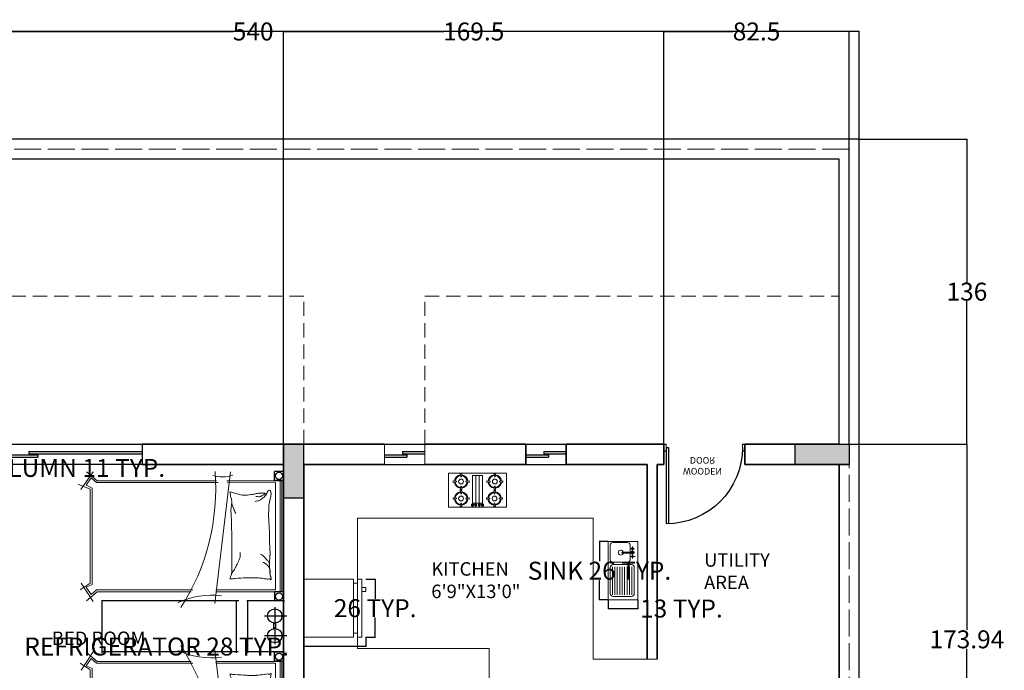
# Model space of a CAD drawing. Units: inches. Extents: x -48 to 50072, y 0 to 21068.
# Tile 71 of 75: x 925 to 1363, y 1005 to 1295. Entities that reach past the tile are written whole.
import ezdxf

# ---------------------------------------------------------------- set-up
doc = ezdxf.new("R2010")
doc.units = ezdxf.units.IN
doc.header["$MEASUREMENT"] = 0
doc.linetypes.add('ACAD_ISO02W100', pattern=[15, 12, -3])
doc.linetypes.add('HIDDEN', pattern=[9.525, 6.35, -3.175])
for name, color, linetype, lineweight in [('A-ANNO-DIMS', 2, 'Continuous', 18), ('A-AREA-IDEN', 7, 'Continuous', 18), ('A-COLS', 1, 'Continuous', 35), ('A-DOOR', 4, 'Continuous', 18), ('A-EQPM', 8, 'Continuous', 18), ('A-FLOR-CASE', 9, 'Continuous', 18), ('A-FLOR-FIXT', 4, 'Continuous', 18), ('A-FLOR-OVHD', 8, 'HIDDEN', 13), ('A-GLAZ', 4, 'Continuous', 18), ('A-WALL', 7, 'Continuous', 35), ('C-PROP', 7, 'Continuous', 25), ('C-PROP-REF', 32, 'ACAD_ISO02W100', 13), ('FURNITURE', 44, 'Continuous', 18)]:
    doc.layers.add(name, color=color, linetype=linetype, lineweight=lineweight)
for name, color, linetype in [('Layer3', 176, 'Continuous'), ('家具1', 1, 'Continuous'), ('家具１', 1, 'Continuous')]:
    doc.layers.add(name, color=color, linetype=linetype)
doc.styles.get("Standard").update_dxf_attribs({"font": 'arial.ttf'})
doc.dimstyles.get("Standard").update_dxf_attribs({"dimtxt": 8, "dimasz": 0.18, "dimexe": 0.18, "dimexo": 0.0625, "dimgap": 0.09, "dimtad": 0, "dimtih": 1, "dimtoh": 1, "dimdec": 1, "dimzin": 0, "dimdsep": 46, "dimlunit": 4, "dimtxsty": 'Standard', "dimblk": 'ARCHTICK', "dimcen": 0.09, "dimadec": 0, "dimazin": 0, "dimtfac": 1, "dimtdec": 1, "dimtofl": 0, "dimtmove": 0, "dimatfit": 3, "dimldrblk": 'ARCHTICK', "dimfxl": 1, "dimtolj": 1, "dimtzin": 0, "dimarcsym": 0})

# ---------------------------------------------------------------- blocks, each defined once
blk = doc.blocks.new('sliding')
blk.add_line((137.02, 1025.77), (137.02, 1034.77))
at = {"layer": 'Defpoints'}
for p, q in [((183.57, 1031.47), (234.12, 1031.47)), ((183.57, 1031.47), (183.57, 1030.47)), ((234.12, 1034.77), (234.12, 1025.77)), ((137.02, 1030.07), (187.57, 1030.07)), ((137.02, 1029.07), (187.57, 1029.07)), ((183.57, 1030.47), (234.12, 1030.47)), ((187.57, 1030.07), (187.57, 1029.07))]:
    blk.add_line(p, q, dxfattribs=at)
at = {"layer": 'Layer3'}
for p, q in [((137.02, 1034.77), (234.12, 1034.77)), ((234.12, 1025.77), (137.02, 1025.77))]:
    blk.add_line(p, q, dxfattribs=at)
blk = doc.blocks.new('bnniku')
at = {"layer": 'Defpoints'}
h = blk.add_hatch(color=256, dxfattribs=at)
h.dxf.hatch_style = 1
h.paths.add_polyline_path([(767.55, 1114.04), (758.55, 1114.04), (758.55, 1090.04), (767.55, 1090.04)])
for p, q in [((758.55, 1114.04), (767.55, 1114.04)), ((758.55, 1090.04), (758.55, 1114.04)), ((767.55, 1114.04), (767.55, 1090.04)), ((767.55, 1090.04), (758.55, 1090.04))]:
    blk.add_line(p, q, dxfattribs=at)
blk = doc.blocks.new('jyugcli')
for p, q in [((342.02, 1025.77), (342.02, 1034.77)), ((360.02, 1025.77), (360.02, 1034.77))]:
    blk.add_line(p, q)
at = {"layer": 'Defpoints'}
for p, q in [((350.02, 1031.47), (360.02, 1031.47)), ((350.02, 1031.47), (350.02, 1030.47)), ((342.02, 1030.07), (352.02, 1030.07)), ((342.02, 1029.07), (352.02, 1029.07)), ((350.02, 1030.47), (360.02, 1030.47)), ((352.02, 1030.07), (352.02, 1029.07))]:
    blk.add_line(p, q, dxfattribs=at)
at = {"layer": 'Layer3'}
for p, q in [((342.02, 1034.77), (360.02, 1034.77)), ((342.02, 1025.77), (360.02, 1025.77))]:
    blk.add_line(p, q, dxfattribs=at)
blk = doc.blocks.new('BKUHJKKUG')
at = {"layer": 'Defpoints'}
for p, q in [((179.52, 862.77), (179.52, 896.77)), ((180.52, 862.77), (180.52, 896.76)), ((179.52, 862.77), (180.52, 862.77))]:
    blk.add_line(p, q, dxfattribs=at)
blk.add_arc((179.52, 862.77), 34, 0, 90, dxfattribs=at)
at = {"insert": (190.84, 874.8), "char_height": 2.9183, "attachment_point": 1}
blk.add_mtext_dynamic_manual_height_columns('\\pxqc;WOODEN ^JDOOR', width=9.6242, gutter_width=14.59, heights=[0], dxfattribs=at)
blk = doc.blocks.new('yfhjudru')
for p, q in [((399.02, 912.27), (399.02, 916.77)), ((435.02, 912.27), (435.02, 916.77)), ((400.02, 912.27), (400.02, 915.27)), ((434.02, 912.27), (434.02, 915.27))]:
    blk.add_line(p, q)
at = {"layer": 'Defpoints'}
for p, q in [((399.02, 915.27), (400.02, 915.27)), ((434.02, 915.27), (435.02, 915.27)), ((399.02, 912.27), (400.02, 912.27)), ((434.02, 912.27), (435.02, 912.27))]:
    blk.add_line(p, q, dxfattribs=at)
blk.add_blockref('BKUHJKKUG', (220.5, 51), dxfattribs=at)
blk = doc.blocks.new('A$C7A8469D8')
for p, q in [((105, 2275), (1345, 2275)), ((105, 1661), (105, 2275)), ((1345, 2255), (105, 2255)), ((1325, 2205), (125, 2205)), ((129, 1663), (125, 2205)), ((1325, 1539), (1325, 2205)), ((1345, 2275), (1345, 1540)), ((3364, 2275), (2124, 2275)), ((2124, 2275), (2124, 1540)), ((2124, 2255), (3364, 2255)), ((2144, 2205), (3344, 2205)), ((2144, 1539), (2144, 2205)), ((3340, 1663), (3344, 2205)), ((3364, 1661), (3364, 2275)), ((997, 2116), (997, 2116)), ((2472, 2116), (2472, 2116)), ((284, 2013), (284, 2013)), ((284, 2013), (284, 2013)), ((941, 2062), (941, 2062)), ((964, 2087), (964, 2087)), ((964, 2087), (964, 2087)), ((2506, 2087), (2506, 2087)), ((2506, 2087), (2506, 2087)), ((2528, 2062), (2528, 2062)), ((3185, 2013), (3185, 2013)), ((3185, 2013), (3185, 2013)), ((240, 1733), (265, 1832)), ((1065, 1762), (1065, 1762)), ((2405, 1762), (2405, 1762)), ((3229, 1733), (3205, 1832)), ((1476, 1525), (6, 1701)), ((231, 1697), (230, 1695)), ((231, 1697), (240, 1733)), ((1097, 1744), (1097, 1744)), ((1097, 1744), (1097, 1744)), ((1097, 1744), (1097, 1744)), ((1993, 1525), (3463, 1701)), ((2372, 1744), (2372, 1744)), ((2372, 1744), (2372, 1744)), ((2372, 1744), (2372, 1744)), ((3238, 1697), (3229, 1733)), ((3238, 1697), (3239, 1695)), ((105, 212), (105, 1543)), ((125, 205), (125, 1562)), ((3344, 205), (3344, 1562)), ((3364, 212), (3364, 1543)), ((1325, 205), (1325, 1280)), ((1345, 1261), (1345, 212)), ((2124, 1261), (2124, 212)), ((2144, 205), (2144, 1280)), ((4, 94), (105, 212)), ((204, 30), (7, 169)), ((125, 205), (73, 144)), ((73, 144), (155, 88)), ((199, 135), (142, 0)), ((155, 88), (187, 155)), ((187, 155), (1264, 155)), ((1251, 135), (199, 135)), ((1453, 169), (1249, 34)), ((1324, 21), (1251, 135)), ((1296, 88), (1264, 155)), ((1378, 144), (1296, 88)), ((1325, 205), (1378, 144)), ((1345, 212), (1446, 92)), ((2017, 169), (2221, 34)), ((2124, 212), (2023, 92)), ((2144, 205), (2092, 144)), ((2092, 144), (2173, 88)), ((2145, 21), (2218, 135)), ((2173, 88), (2205, 155)), ((3282, 155), (2205, 155)), ((2218, 135), (3270, 135)), ((3265, 30), (3463, 169)), ((3270, 135), (3328, 0)), ((3315, 88), (3282, 155)), ((3396, 144), (3315, 88)), ((3344, 205), (3396, 144)), ((3465, 94), (3364, 212))]:
    blk.add_line(p, q)
for centre, radius, start, end in [((227, 2136), 15.7, 101.2724, 206.5805), ((250, 2148), 41, 206.5805, 265.5998), ((245, 2045), 108, 90, 101.2724), ((833, 2043), 590, 173.7676, 180), ((245, 1961), 193, 81.5628, 90), ((170, 1957), 168, 45.0976, 62.7964), ((220, 1790), 366, 74.256, 81.5628), ((398, 2422), 291, 254.256, 262.4531), ((468, 2946), 819, 262.4531, 270), ((468, 3385), 1259, 270, 276.0867), ((201, 24611), 22481, 271.0184, 271.708), ((904, 1960), 183, 92.5386, 100.1899), ((911, 1796), 348, 85.1982, 92.5386), ((1028, 3186), 1048, 265.1982, 269.4243), ((1289, 1747), 470, 128.3886, 133.8115), ((1289, 1747), 470, 128.3886, 133.8115), ((1289, 1747), 470, 128.3886, 133.8115), ((1054, 2044), 92.1, 117.2396, 128.3886), ((1141, 1876), 281, 110.8603, 117.2396), ((1035, 3931), 1793, 269.4243, 271.9079), ((1130, 2026), 119, 143.8234, 161.5603), ((1130, 2026), 119, 126.0864, 143.8234), ((1130, 2026), 119, 105.9352, 126.0864), ((1062, 3124), 985, 271.9079, 275.2592), ((1130, 2026), 119, 85.7841, 105.9352), ((1147, 2207), 64.7, 275.2592, 300.6513), ((1197, 2122), 34.7, 85.6975, 120.6513), ((1434, 2041), 238, 167.8905, 172.3191), ((1198, 2126), 30.1, 68.2117, 85.6975), ((1220, 2138), 18.7, 158.0096, 201.421), ((912, 2153), 295, 347.8905, 351.8665), ((1207, 2143), 5.13, 78.1069, 158.0096), ((1166, 2117), 39.3, 351.8665, 21.421), ((1209, 2151), 2.78, 258.1069, 19.564), ((1207, 2150), 4.1, 19.564, 68.2117), ((2257, 2156), 4.1, 291.7883, 340.436), ((2259, 2149), 2.78, 340.436, 101.8931), ((2258, 2184), 30.1, 274.3025, 291.7883), ((2266, 2150), 5.13, 201.9904, 281.8931), ((2228, 2126), 39.3, 338.579, 8.1335), ((1976, 2049), 295, 8.1335, 12.1095), ((2284, 2138), 18.7, 158.579, 201.9904), ((2504, 2123), 238, 187.6809, 192.1095), ((2287, 2186), 34.7, 239.3487, 274.3025), ((2284, 2087), 64.7, 59.3487, 84.7408), ((2284, 1158), 985, 84.7408, 88.0921), ((2363, 2260), 119, 254.0648, 274.2159), ((2442, 2237), 119, 233.9136, 254.0648), ((2392, 346), 1793, 88.0921, 90.5757), ((2505, 2193), 119, 216.1766, 233.9136), ((2557, 2388), 281, 242.7604, 249.1397), ((2548, 2134), 119, 198.4397, 216.1766), ((2540, 1094), 1048, 90.5757, 94.8018), ((2514, 2198), 92.1, 231.6114, 242.7604), ((2798, 2455), 470, 226.1885, 231.6114), ((2180, 1747), 470, 46.1885, 51.6114), ((2180, 1747), 470, 46.1885, 51.6114), ((2544, 2489), 348, 267.4614, 274.8018), ((2606, 2323), 183, 259.8101, 267.4614), ((2198, -20338), 22481, 88.292, 88.9816), ((2868, 875), 1259, 83.9133, 90), ((3109, 1314), 819, 90, 97.5469), ((3188, 1854), 291, 97.5469, 105.744), ((3096, 2504), 366, 278.4372, 285.744), ((3104, 2226), 168, 297.2036, 314.9024), ((3196, 2345), 193, 270, 278.4372), ((3259, 2088), 41, 94.4002, 153.4195), ((3813, 2107), 590, 180, 186.2324), ((3245, 2260), 108, 258.7276, 270), ((3259, 2145), 15.7, 153.4195, 258.7276), ((488, 2043), 245, 180, 189.6844), ((181, 2001), 108, 41.4429, 53.7359), ((1290, 2180), 1058, 189.6844, 192.1984), ((214, 2030), 63.1, 25.3551, 41.4429), ((108, 1980), 181, 21.8149, 25.3551), ((47, 1955), 247, 18.7799, 21.8149), ((217, 2013), 67.4, 0, 18.7799), ((174, 2013), 110, 345.3149, 360), ((170, 1957), 168, 27.3988, 45.0976), ((170, 1957), 168, 16.515, 27.3988), ((170, 1957), 168, 5.6311, 16.515), ((1146, 1939), 240, 151.6832, 156.9972), ((987, 2024), 59.2, 140.9651, 151.6832), ((1151, 1892), 270, 133.8115, 140.9651), ((1151, 1892), 270, 133.8115, 140.9651), ((1151, 1892), 270, 133.8115, 140.9651), ((2003, 1943), 814, 176.6313, 181.6331), ((2284, 1927), 1096, 172.3191, 176.6313), ((3365, 2137), 1096, 183.3687, 187.6809), ((3094, 1968), 814, 178.3669, 183.3687), ((2716, 2257), 270, 219.0349, 226.1885), ((2319, 1892), 270, 39.0349, 46.1885), ((2319, 1892), 270, 39.0349, 46.1885), ((2581, 2090), 59.2, 208.3168, 219.0349), ((2756, 2146), 240, 203.0028, 208.3168), ((2972, 2022), 168, 343.485, 354.3689), ((2990, 2082), 168, 332.6012, 343.485), ((3032, 2154), 168, 314.9024, 332.6012), ((3121, 2035), 67.4, 341.2201, 360), ((3079, 1985), 110, 0, 14.6851), ((2960, 2126), 247, 338.1851, 341.2201), ((3030, 2125), 181, 334.6449, 338.1851), ((3151, 2099), 63.1, 318.5571, 334.6449), ((3144, 2159), 108, 306.2641, 318.5571), ((4257, 1778), 1058, 167.8016, 170.3156), ((3468, 2002), 245, 170.3156, 180), ((-117, 1876), 381, 8.0051, 12.1984), ((-523, 1819), 791, 2.6649, 8.0051), ((2826, 1967), 1638, 181.6331, 183.055), ((17530, 2751), 16363, 183.055, 183.5049), ((18611, 879), 16363, 176.4951, 176.945), ((3917, 1833), 1638, 176.945, 178.3669), ((2419, 1966), 791, 351.9949, 357.3351), ((2837, 2009), 381, 347.8016, 351.9949), ((186, 1852), 81.3, 345.9548, 2.6649), ((93, 2561), 886, 293.4844, 295.3111), ((927, 1484), 326, 85.9172, 93.5552), ((946, 1740), 69.6, 69.3257, 85.9172), ((755, 1236), 608, 65.6735, 69.3257), ((298, 224), 1719, 63.5015, 65.6735), ((897, 1427), 375, 57.865, 63.5015), ((897, 1427), 375, 57.865, 63.5015), ((897, 1427), 375, 57.865, 63.5015), ((2205, 2080), 375, 296.4985, 302.135), ((2572, 1427), 375, 116.4985, 122.135), ((2572, 1427), 375, 116.4985, 122.135), ((1697, 3328), 1719, 294.3265, 296.4985), ((2249, 2359), 608, 290.6743, 294.3265), ((2494, 1874), 69.6, 274.0828, 290.6743), ((2539, 2135), 326, 266.4448, 274.0828), ((2644, 947), 886, 64.6889, 66.5156), ((3123, 1836), 81.3, 357.3351, 14.0452), ((-288, 1612), 350, 341.9888, 19.1136), ((209, 2020), 325, 273.8155, 274.0829), ((232, 1697), 1.1, 165.9546, 274.0829), ((232, 1697), 1.1, 165.9551, 274.0829), ((209, 2020), 325, 274.0829, 279.4841), ((217, 1971), 276, 279.4841, 287.3864), ((342, 1571), 144, 96.4341, 107.3864), ((346, 1540), 175, 78.4414, 96.4341), ((93, 2561), 886, 287.1982, 289.428), ((436, 1982), 276, 258.4414, 272.7491), ((93, 2561), 886, 289.4267, 291.8864), ((93, 2561), 886, 289.4283, 291.559), ((93, 2561), 886, 289.428, 291.6577), ((93, 2561), 886, 289.4267, 289.4283), ((93, 2561), 886, 291.443, 291.8345), ((93, 2561), 886, 291.43, 291.71), ((93, 2561), 886, 291.43, 291.7259), ((93, 2561), 886, 291.443, 291.484), ((93, 2561), 886, 291.484, 291.7259), ((93, 2561), 886, 291.559, 291.8345), ((93, 2561), 886, 291.6577, 293.4844), ((93, 2561), 886, 291.71, 291.8864), ((369, 3390), 1686, 272.7491, 274.6176), ((622, 254), 1460, 92.6096, 94.6176), ((1098, -33471), 35188, 90.3285, 90.8836), ((1012, -5145), 6862, 89.7135, 90.9704), ((1040, 320), 1397, 86.426, 89.7135), ((632, 1004), 874, 54.1737, 57.865), ((1116, 1540), 175, 77.131, 86.426), ((1143, 1657), 54.3, 62.7159, 77.131), ((1210, 1788), 92.1, 242.7159, 253.7788), ((1214, 1800), 105, 253.7788, 262.8796), ((1582, 1775), 385, 183.5049, 189.9984), ((1201, 1697), 1.59, 262.8796, 343.3022), ((1180, 1704), 23.2, 343.3022, 9.9984), ((2651, 1684), 385, 170.0016, 176.4951), ((2244, 1701), 23.2, 350.0016, 16.6978), ((2267, 1695), 1.59, 16.6978, 97.1204), ((2298, 1595), 105, 97.1204, 106.2212), ((2327, 1617), 92.1, 106.2212, 117.2841), ((2289, 1759), 54.3, 282.869, 297.2841), ((2303, 1885), 175, 273.574, 282.869), ((1861, 2453), 874, 302.135, 305.8263), ((2335, 3111), 1397, 270.2865, 273.574), ((2539, 8578), 6862, 269.0296, 270.2865), ((3116, 36900), 35188, 269.1164, 269.6715), ((3031, 3168), 1460, 265.3824, 267.3904), ((2884, 26), 1686, 85.3824, 87.2509), ((3075, 1435), 276, 87.2509, 101.5586), ((2696, 925), 886, 66.5156, 68.3423), ((3376, 2561), 886, 248.1136, 250.5733), ((3376, 2561), 886, 248.1136, 248.29), ((3376, 2561), 886, 248.1655, 248.557), ((3376, 2561), 886, 248.1655, 248.441), ((3376, 2561), 886, 248.29, 248.57), ((3376, 2561), 886, 248.2741, 248.57), ((3376, 2561), 886, 248.2741, 248.516), ((2754, 902), 886, 68.3423, 70.572), ((3376, 2561), 886, 248.441, 250.5717), ((3376, 2561), 886, 248.516, 248.557), ((3376, 2561), 886, 250.5717, 250.5733), ((2819, 879), 886, 70.572, 72.8018), ((3108, 1885), 175, 263.5659, 281.5586), ((3186, 1851), 144, 252.6136, 263.5659), ((3125, 1436), 276, 72.6136, 80.5159), ((3184, 1375), 325, 80.5159, 85.9171), ((3237, 1697), 1.1, 265.9171, 14.0454), ((3238, 1696), 1.1, 85.9171, 194.0449), ((3260, 2020), 325, 265.9171, 266.1845), ((3757, 1612), 350, 160.8864, 198.0112), ((2297, 1493), 913, 173.1442, 204.7336), ((1172, 1493), 913, 335.2664, 6.8558), ((192, -937), 2473, 57.4247, 94.4416), ((3278, -937), 2473, 85.5584, 122.5753)]:
    blk.add_arc(centre, radius, start, end)
at = {"layer": '家具1'}
for p, q in [((1614, 2082), (1614, 2330)), ((1836, 2082), (1836, 2330)), ((101, 2293), (1, 2293)), ((1, 2293), (1, 2193)), ((101, 2293), (101, 2193)), ((1348, 2293), (1448, 2293)), ((1348, 2293), (1348, 2193)), ((2032, 2293), (1441, 2293)), ((1448, 2303), (1448, 1885)), ((1448, 2293), (1448, 2193)), ((1757, 2206), (1696, 2206)), ((2018, 2303), (2018, 1885)), ((2121, 2293), (2021, 2293)), ((2021, 2293), (2021, 2193)), ((2121, 2293), (2121, 2193)), ((3369, 2293), (3469, 2293)), ((3369, 2293), (3369, 2193)), ((101, 2193), (1, 2193)), ((1348, 2193), (1448, 2193)), ((1518, 2197), (1709, 2197)), ((1757, 2186), (1696, 2186)), ((1741, 2197), (1931, 2197)), ((2121, 2193), (2021, 2193)), ((3369, 2193), (3469, 2193)), ((2029, 1893), (1441, 1893)), ((2029, 1768), (1441, 1768)), ((1448, 1793), (1448, 260)), ((2018, 1788), (2018, 260)), ((2029, 268), (1441, 268))]:
    blk.add_line(p, q, dxfattribs=at)
for centre, radius in [((51, 2243), 40), ((1398, 2243), 40), ((1616, 2196), 80), ((1836, 2196), 80), ((2071, 2243), 40), ((3419, 2243), 40)]:
    blk.add_circle(centre, radius, dxfattribs=at)
at = {"layer": '家具１'}
blk.add_line((3469, 2293), (3469, 2193), dxfattribs=at)
blk = doc.blocks.new('A$C593E77E4')
for p, q in [((0, 0), (0, 0.911)), ((0, 0.911), (1.781, 0.911)), ((1.781, 0), (1.781, 0.911)), ((0.321, 0.668), (0.105, 0.668)), ((0.279, 0.745, -0.922), (0.15, 0.745, -0.922)), ((0.216, 0.808, -0.922), (0.216, 0.672, -0.922)), ((0.321, 0.784, -0.922), (0.321, 0.434, -0.922)), ((0.349, 0.784, -0.922), (0.321, 0.784, -0.922)), ((0.349, 0.434, -0.922), (0.349, 0.784, -0.922)), ((0.555, 0.668), (0.349, 0.668)), ((0.39, 0.745, -0.922), (0.519, 0.745, -0.922)), ((0.455, 0.826, -0.922), (0.455, 0.689, -0.922)), ((0.705, 0.706), (0.705, 0.158)), ((0.772, 0.729, 1.373), (1.625, 0.729, 1.373)), ((0.772, 0.654, 1.373), (1.625, 0.654, 1.373)), ((1.588, 0.797), (0.797, 0.797)), ((1.68, 0.158), (1.68, 0.706)), ((0.03, 0.593), (0.03, 0.141)), ((0.63, 0.141), (0.63, 0.593)), ((0.772, 0.579, 1.373), (1.625, 0.579, 1.373)), ((0.772, 0.504, 1.373), (1.625, 0.504, 1.373)), ((0.772, 0.429, 1.373), (1.625, 0.429, 1.373)), ((0.772, 0.354, 1.373), (1.625, 0.354, 1.373)), ((0.105, 0.066), (0.555, 0.066)), ((0.772, 0.279, 1.373), (1.625, 0.279, 1.373)), ((0.772, 0.204, 1.373), (1.625, 0.204, 1.373)), ((0.772, 0.129, 1.373), (1.625, 0.129, 1.373)), ((0.797, 0.066), (1.588, 0.066)), ((1.781, 0), (0, 0))]:
    blk.add_line(p, q)
for centre in [(0.216, 0.745, -0.922), (0.454, 0.745, -0.922)]:
    blk.add_circle(centre, 0.0299)
for centre, radius, start, end in [((0.105, 0.593), 0.075, 90, 180), ((0.333, 0.75, -0.922), 0.0447, 290.1713, 253.9866), ((0.555, 0.593), 0.075, 0, 90), ((0.797, 0.706), 0.0919, 90, 180), ((1.588, 0.706), 0.0919, 0, 90), ((0.336, 0.387, 0.688), 0.0774, 101.239, 83.3158), ((0.335, 0.435, -0.922), 0.0139, 185.1203, 354.8797), ((0.105, 0.141), 0.075, 180, 270), ((0.555, 0.141), 0.075, 270, 0), ((0.797, 0.158), 0.0919, 180, 270), ((1.588, 0.158), 0.0919, 270, 0)]:
    blk.add_arc(centre, radius, start, end)
blk = doc.blocks.new('A$C57CF26DA')
for p, q in [((0, 0), (0, 420)), ((720, 420), (0, 420)), ((167, 413), (147, 413)), ((147, 413), (152, 373)), ((152, 373), (162, 373)), ((162, 373), (167, 413)), ((300, 391), (300, 49)), ((300, 391), (420, 391)), ((340, 391), (340, 49)), ((380, 391), (380, 49)), ((420, 391), (420, 49)), ((584, 413), (564, 413)), ((564, 413), (569, 373)), ((569, 373), (579, 373)), ((579, 373), (584, 413)), ((720, 0), (720, 420)), ((99, 320), (59, 325)), ((59, 325), (59, 305)), ((59, 305), (99, 310)), ((99, 310), (99, 320)), ((152, 257), (147, 217)), ((162, 257), (152, 257)), ((167, 217), (162, 257)), ((255, 325), (215, 320)), ((215, 320), (215, 310)), ((215, 310), (255, 305)), ((255, 305), (255, 325)), ((516, 320), (476, 325)), ((476, 325), (476, 305)), ((476, 305), (516, 310)), ((516, 310), (516, 320)), ((569, 257), (564, 217)), ((579, 257), (569, 257)), ((584, 217), (579, 257)), ((672, 325), (632, 320)), ((632, 320), (632, 310)), ((632, 310), (672, 305)), ((672, 305), (672, 325)), ((147, 217), (167, 217)), ((167, 203), (147, 203)), ((147, 203), (152, 163)), ((152, 163), (162, 163)), ((162, 163), (167, 203)), ((581, 203), (561, 203)), ((561, 203), (566, 163)), ((564, 217), (584, 217)), ((566, 163), (576, 163)), ((576, 163), (581, 203)), ((99, 110), (59, 115)), ((59, 115), (59, 95)), ((59, 95), (99, 100)), ((99, 100), (99, 110)), ((152, 47), (147, 7)), ((147, 7), (167, 7)), ((162, 47), (152, 47)), ((167, 7), (162, 47)), ((255, 115), (215, 110)), ((215, 110), (215, 100)), ((215, 100), (255, 95)), ((255, 95), (255, 115)), ((302, 39), (295, 39)), ((295, 39), (295, 11)), ((295, 11), (302, 11)), ((420, 49), (300, 49)), ((302, 11), (302, 39)), ((341, 39), (334, 39)), ((334, 39), (334, 11)), ((334, 11), (341, 11)), ((341, 11), (341, 39)), ((380, 11), (380, 39)), ((380, 39), (386, 39)), ((386, 11), (380, 11)), ((386, 39), (386, 11)), ((419, 11), (419, 39)), ((419, 39), (426, 39)), ((426, 11), (419, 11)), ((426, 39), (426, 11)), ((513, 110), (473, 115)), ((473, 115), (473, 95)), ((473, 95), (513, 100)), ((513, 100), (513, 110)), ((566, 47), (561, 7)), ((561, 7), (581, 7)), ((576, 47), (566, 47)), ((581, 7), (576, 47)), ((669, 115), (629, 110)), ((629, 110), (629, 100)), ((629, 100), (669, 95)), ((669, 95), (669, 115)), ((720, 0), (0, 0))]:
    blk.add_line(p, q)
for centre in [(157, 315), (574, 315), (157, 105), (571, 105)]:
    blk.add_circle(centre, 30)
for centre, radius, start, end in [((157, 315), 83, 95.5849, 174.4151), ((157, 315), 73, 95.3738, 174.6262), ((157, 315), 73, 5.3738, 84.6262), ((157, 315), 83, 5.5849, 84.4151), ((574, 315), 83, 95.5849, 174.4151), ((574, 315), 73, 95.3738, 174.6262), ((574, 315), 73, 5.3738, 84.6262), ((574, 315), 83, 5.5849, 84.4151), ((157, 315), 83, 185.5849, 264.4151), ((157, 315), 73, 185.3738, 264.6262), ((157, 315), 73, 275.3738, 354.6262), ((157, 315), 83, 275.5849, 354.4151), ((574, 315), 83, 185.5849, 264.4151), ((574, 315), 73, 185.3738, 264.6262), ((574, 315), 73, 275.3738, 354.6262), ((574, 315), 83, 275.5849, 354.4151), ((157, 105), 83, 95.5849, 174.4151), ((157, 105), 73, 95.3738, 174.6262), ((157, 105), 73, 5.3738, 84.6262), ((157, 105), 83, 5.5849, 84.4151), ((571, 105), 83, 95.5849, 174.4151), ((571, 105), 73, 95.3738, 174.6262), ((571, 105), 73, 5.3738, 84.6262), ((571, 105), 83, 5.5849, 84.4151), ((157, 105), 83, 185.5849, 264.4151), ((157, 105), 73, 185.3738, 264.6262), ((157, 105), 73, 275.3738, 354.6262), ((157, 105), 83, 275.5849, 354.4151), ((298, 25), 13.7, 104.4775, 255.5225), ((298, 25), 13.7, 284.4775, 75.5225), ((337, 25), 13.7, 104.4775, 255.5225), ((337, 25), 13.7, 284.4775, 75.5225), ((383, 25), 13.7, 104.4775, 255.5225), ((383, 25), 13.7, 284.4775, 75.5225), ((422, 25), 13.7, 104.4775, 255.5225), ((422, 25), 13.7, 284.4775, 75.5225), ((571, 105), 83, 185.5849, 264.4151), ((571, 105), 73, 185.3738, 264.6262), ((571, 105), 73, 275.3738, 354.6262), ((571, 105), 83, 275.5849, 354.4151)]:
    blk.add_arc(centre, radius, start, end)
blk = doc.blocks.new('REFRI-00')
for points in [[(-0.35, 0.35), (-0.35, -0.25), (0.35, -0.25), (0.35, 0.35), (-0.35, 0.35)], [(-0.35, -0.3), (-0.35, -0.35), (0.35, -0.35), (0.35, -0.3), (-0.35, -0.3)], [(-0.3, -0.3), (-0.3, -0.25)], [(-0.25, -0.35), (-0.25, -0.4), (-0.2, -0.4), (-0.2, -0.35)], [(0.3, -0.3), (0.3, -0.25)]]:
    blk.add_lwpolyline(points)
blk = doc.blocks.new('_ArchTick')
at = {"color": 0, "linetype": 'ByBlock', "const_width": 0.15}
blk.add_lwpolyline([(-0.5, -0.5), (0.5, 0.5)], dxfattribs=at)
blk = doc.blocks.new('*D50')
at = {"layer": 'A-ANNO-DIMS', "color": 0, "lineweight": -2, "transparency": 16777216}
for p, q in [((850.76, 1096.4), (850.76, 1094.71)), ((850.76, 1094.89), (861.26, 1094.89)), ((861.26, 1096.4), (861.26, 1094.71)), ((861.26, 1094.89), (861.44, 1094.89))]:
    blk.add_line(p, q, dxfattribs=at)
at = {"layer": 'Defpoints', "color": 0, "transparency": 16777216}
for p in [(850.76, 1096.46), (861.26, 1096.46), (861.26, 1094.89)]:
    blk.add_point(p, dxfattribs=at)
at = {"layer": 'A-ANNO-DIMS', "color": 0, "lineweight": -2, "transparency": 16777216, "xscale": 0.18, "yscale": 0.18, "zscale": 0.18, "rotation": 180}
blk.add_blockref('_ArchTick', (850.76, 1094.89), dxfattribs=at)
at = {"layer": 'A-ANNO-DIMS', "color": 0, "lineweight": -2, "transparency": 16777216, "xscale": 0.18, "yscale": 0.18, "zscale": 0.18}
blk.add_blockref('_ArchTick', (861.26, 1094.89), dxfattribs=at)
at = {"layer": 'A-ANNO-DIMS', "color": 0, "transparency": 16777216, "insert": (927.86, 1094.89), "char_height": 8, "attachment_point": 5}
blk.add_mtext('\\A1;SHORT COLUMN 11 TYP.', dxfattribs=at)
blk = doc.blocks.new('*D88')
at = {"layer": 'A-ANNO-DIMS', "color": 0, "lineweight": -2, "transparency": 16777216}
for p, q in [((1186.84, 1062.05), (1182.84, 1062.05)), ((1183.02, 1062.05), (1183.02, 1053.31)), ((1183.02, 1036.11), (1183.02, 1044.85)), ((1186.84, 1036.11), (1182.84, 1036.11))]:
    blk.add_line(p, q, dxfattribs=at)
at = {"layer": 'Defpoints', "color": 0, "transparency": 16777216}
for p in [(1186.91, 1062.05), (1183.02, 1036.11), (1186.91, 1036.11)]:
    blk.add_point(p, dxfattribs=at)
at = {"layer": 'A-ANNO-DIMS', "color": 0, "lineweight": -2, "transparency": 16777216, "xscale": 0.18, "yscale": 0.18, "zscale": 0.18}
for p, rotation in [((1183.02, 1062.05), 90), ((1183.02, 1036.11), 270)]:
    blk.add_blockref('_ArchTick', p, dxfattribs=dict(at, rotation=rotation))
at = {"layer": 'A-ANNO-DIMS', "color": 0, "transparency": 16777216, "insert": (1183.02, 1049.08), "char_height": 8, "attachment_point": 5}
blk.add_mtext('\\A1;SINK 26 TYP.', dxfattribs=at)
blk = doc.blocks.new('*D89')
at = {"layer": 'A-ANNO-DIMS', "color": 0, "lineweight": -2, "transparency": 16777216}
for p, q in [((1186.91, 1036.05), (1186.91, 1032.04)), ((1200.16, 1036.05), (1200.16, 1032.04)), ((1186.91, 1032.22), (1200.16, 1032.22)), ((1200.16, 1032.22), (1200.34, 1032.22))]:
    blk.add_line(p, q, dxfattribs=at)
at = {"layer": 'Defpoints', "color": 0, "transparency": 16777216}
for p in [(1186.91, 1036.11), (1200.16, 1036.11), (1200.16, 1032.22)]:
    blk.add_point(p, dxfattribs=at)
at = {"layer": 'A-ANNO-DIMS', "color": 0, "lineweight": -2, "transparency": 16777216, "xscale": 0.18, "yscale": 0.18, "zscale": 0.18, "rotation": 180}
blk.add_blockref('_ArchTick', (1186.91, 1032.22), dxfattribs=at)
at = {"layer": 'A-ANNO-DIMS', "color": 0, "lineweight": -2, "transparency": 16777216, "xscale": 0.18, "yscale": 0.18, "zscale": 0.18}
blk.add_blockref('_ArchTick', (1200.16, 1032.22), dxfattribs=at)
at = {"layer": 'A-ANNO-DIMS', "color": 0, "transparency": 16777216, "insert": (1219.53, 1032.22), "char_height": 8, "attachment_point": 5}
blk.add_mtext('\\A1;13 TYP.', dxfattribs=at)
blk = doc.blocks.new('*D92')
at = {"layer": 'A-ANNO-DIMS', "color": 0, "lineweight": -2, "transparency": 16777216}
for p, q in [((1051.25, 1019.39), (1051.25, 1015.11)), ((1078.96, 1019.39), (1078.96, 1015.11)), ((1051.25, 1015.29), (1051.07, 1015.29)), ((1078.96, 1015.29), (1051.25, 1015.29))]:
    blk.add_line(p, q, dxfattribs=at)
at = {"layer": 'Defpoints', "color": 0, "transparency": 16777216}
for p in [(1051.25, 1019.45), (1078.96, 1019.45), (1051.25, 1015.29)]:
    blk.add_point(p, dxfattribs=at)
at = {"layer": 'A-ANNO-DIMS', "color": 0, "lineweight": -2, "transparency": 16777216, "xscale": 0.18, "yscale": 0.18, "zscale": 0.18, "rotation": 180}
blk.add_blockref('_ArchTick', (1051.25, 1015.29), dxfattribs=at)
at = {"layer": 'A-ANNO-DIMS', "color": 0, "lineweight": -2, "transparency": 16777216, "xscale": 0.18, "yscale": 0.18, "zscale": 0.18}
blk.add_blockref('_ArchTick', (1078.96, 1015.29), dxfattribs=at)
at = {"layer": 'A-ANNO-DIMS', "color": 0, "transparency": 16777216, "insert": (985.76, 1015.29), "char_height": 8, "attachment_point": 5}
blk.add_mtext('\\A1;REFRIGERATOR 28 TYP.', dxfattribs=at)
blk = doc.blocks.new('*D93')
at = {"layer": 'A-ANNO-DIMS', "color": 0, "lineweight": -2, "transparency": 16777216}
for p, q in [((1079.02, 1045.31), (1083.29, 1045.31)), ((1083.11, 1045.31), (1083.11, 1036.55)), ((1083.11, 1019.45), (1083.11, 1028.21)), ((1079.02, 1019.45), (1083.29, 1019.45))]:
    blk.add_line(p, q, dxfattribs=at)
at = {"layer": 'Defpoints', "color": 0, "transparency": 16777216}
for p in [(1078.96, 1045.31), (1078.96, 1019.45), (1083.11, 1019.45)]:
    blk.add_point(p, dxfattribs=at)
at = {"layer": 'A-ANNO-DIMS', "color": 0, "lineweight": -2, "transparency": 16777216, "xscale": 0.18, "yscale": 0.18, "zscale": 0.18}
for p, rotation in [((1083.11, 1045.31), 90), ((1083.11, 1019.45), 270)]:
    blk.add_blockref('_ArchTick', p, dxfattribs=dict(at, rotation=rotation))
at = {"layer": 'A-ANNO-DIMS', "color": 0, "transparency": 16777216, "insert": (1083.11, 1032.38), "char_height": 8, "attachment_point": 5}
blk.add_mtext('\\A1;26 TYP.', dxfattribs=at)
blk = doc.blocks.new('*D129')
at = {"layer": 'A-ANNO-DIMS', "color": 0, "lineweight": -2, "transparency": 16777216}
for p, q in [((758.76, 1241.53), (758.76, 1289.59)), ((1298.76, 1241.53), (1298.76, 1289.59)), ((758.76, 1289.41), (1019.85, 1289.41)), ((1298.76, 1289.41), (1037.67, 1289.41))]:
    blk.add_line(p, q, dxfattribs=at)
at = {"layer": 'Defpoints', "color": 0, "transparency": 16777216}
for p in [(1298.76, 1289.41), (758.76, 1241.46), (1298.76, 1241.46)]:
    blk.add_point(p, dxfattribs=at)
at = {"layer": 'A-ANNO-DIMS', "color": 0, "lineweight": -2, "transparency": 16777216, "xscale": 0.18, "yscale": 0.18, "zscale": 0.18, "rotation": 180}
blk.add_blockref('_ArchTick', (758.76, 1289.41), dxfattribs=at)
at = {"layer": 'A-ANNO-DIMS', "color": 0, "lineweight": -2, "transparency": 16777216, "xscale": 0.18, "yscale": 0.18, "zscale": 0.18}
blk.add_blockref('_ArchTick', (1298.76, 1289.41), dxfattribs=at)
at = {"layer": 'A-ANNO-DIMS', "color": 0, "transparency": 16777216, "insert": (1028.76, 1289.41), "char_height": 8, "attachment_point": 5}
blk.add_mtext('\\A1;540', dxfattribs=at)
blk = doc.blocks.new('*D131')
at = {"layer": 'A-ANNO-DIMS', "color": 0, "lineweight": -2, "transparency": 16777216}
for p, q in [((1298.82, 1241.46), (1346.89, 1241.46)), ((1346.71, 1241.46), (1346.71, 1177.64)), ((1346.71, 1105.46), (1346.71, 1169.29)), ((1294.32, 1105.46), (1346.89, 1105.46))]:
    blk.add_line(p, q, dxfattribs=at)
at = {"layer": 'Defpoints', "color": 0, "transparency": 16777216}
for p in [(1298.76, 1241.46), (1294.26, 1105.46), (1346.71, 1105.46)]:
    blk.add_point(p, dxfattribs=at)
at = {"layer": 'A-ANNO-DIMS', "color": 0, "lineweight": -2, "transparency": 16777216, "xscale": 0.18, "yscale": 0.18, "zscale": 0.18}
for p, rotation in [((1346.71, 1241.46), 90), ((1346.71, 1105.46), 270)]:
    blk.add_blockref('_ArchTick', p, dxfattribs=dict(at, rotation=rotation))
at = {"layer": 'A-ANNO-DIMS', "color": 0, "transparency": 16777216, "insert": (1346.71, 1173.46), "char_height": 8, "attachment_point": 5}
blk.add_mtext('\\A1;136', dxfattribs=at)
blk = doc.blocks.new('*D133')
at = {"layer": 'A-ANNO-DIMS', "color": 0, "lineweight": -2, "transparency": 16777216}
for p, q in [((1294.32, 1105.46), (1346.89, 1105.46)), ((1346.71, 1105.46), (1346.71, 1022.67)), ((1346.71, 931.53), (1346.71, 1014.32)), ((1294.32, 931.53), (1346.89, 931.53))]:
    blk.add_line(p, q, dxfattribs=at)
at = {"layer": 'Defpoints', "color": 0, "transparency": 16777216}
for p in [(1294.26, 1105.46), (1294.26, 931.53), (1346.71, 931.53)]:
    blk.add_point(p, dxfattribs=at)
at = {"layer": 'A-ANNO-DIMS', "color": 0, "lineweight": -2, "transparency": 16777216, "xscale": 0.18, "yscale": 0.18, "zscale": 0.18}
for p, rotation in [((1346.71, 1105.46), 90), ((1346.71, 931.53), 270)]:
    blk.add_blockref('_ArchTick', p, dxfattribs=dict(at, rotation=rotation))
at = {"layer": 'A-ANNO-DIMS', "color": 0, "transparency": 16777216, "insert": (1346.71, 1018.5), "char_height": 8, "attachment_point": 5}
blk.add_mtext('\\A1;173.94', dxfattribs=at)
blk = doc.blocks.new('*D142')
at = {"layer": 'A-ANNO-DIMS', "color": 0, "lineweight": -2, "transparency": 16777216}
for p, q in [((763.26, 1105.53), (763.26, 1289.59)), ((1042.26, 1105.53), (1042.26, 1289.59)), ((763.26, 1289.41), (893.76, 1289.41)), ((1042.26, 1289.41), (911.76, 1289.41))]:
    blk.add_line(p, q, dxfattribs=at)
at = {"layer": 'Defpoints', "color": 0, "transparency": 16777216}
for p in [(1042.26, 1289.41), (763.26, 1105.46), (1042.26, 1105.46)]:
    blk.add_point(p, dxfattribs=at)
at = {"layer": 'A-ANNO-DIMS', "color": 0, "lineweight": -2, "transparency": 16777216, "xscale": 0.18, "yscale": 0.18, "zscale": 0.18, "rotation": 180}
blk.add_blockref('_ArchTick', (763.26, 1289.41), dxfattribs=at)
at = {"layer": 'A-ANNO-DIMS', "color": 0, "lineweight": -2, "transparency": 16777216, "xscale": 0.18, "yscale": 0.18, "zscale": 0.18}
blk.add_blockref('_ArchTick', (1042.26, 1289.41), dxfattribs=at)
at = {"layer": 'A-ANNO-DIMS', "color": 0, "transparency": 16777216, "insert": (902.76, 1289.41), "char_height": 8, "attachment_point": 5}
blk.add_mtext('\\A1;279', dxfattribs=at)
blk = doc.blocks.new('*D143')
at = {"layer": 'A-ANNO-DIMS', "color": 0, "lineweight": -2, "transparency": 16777216}
for p, q in [((1042.26, 1105.53), (1042.26, 1289.59)), ((1211.76, 1105.53), (1211.76, 1289.59)), ((1042.26, 1289.41), (1113.77, 1289.41)), ((1211.76, 1289.41), (1140.25, 1289.41))]:
    blk.add_line(p, q, dxfattribs=at)
at = {"layer": 'Defpoints', "color": 0, "transparency": 16777216}
for p in [(1211.76, 1289.41), (1042.26, 1105.46), (1211.76, 1105.46)]:
    blk.add_point(p, dxfattribs=at)
at = {"layer": 'A-ANNO-DIMS', "color": 0, "lineweight": -2, "transparency": 16777216, "xscale": 0.18, "yscale": 0.18, "zscale": 0.18, "rotation": 180}
blk.add_blockref('_ArchTick', (1042.26, 1289.41), dxfattribs=at)
at = {"layer": 'A-ANNO-DIMS', "color": 0, "lineweight": -2, "transparency": 16777216, "xscale": 0.18, "yscale": 0.18, "zscale": 0.18}
blk.add_blockref('_ArchTick', (1211.76, 1289.41), dxfattribs=at)
at = {"layer": 'A-ANNO-DIMS', "color": 0, "transparency": 16777216, "insert": (1127.01, 1289.41), "char_height": 8, "attachment_point": 5}
blk.add_mtext('\\A1;169.5', dxfattribs=at)
blk = doc.blocks.new('*D144')
at = {"layer": 'A-ANNO-DIMS', "color": 0, "lineweight": -2, "transparency": 16777216}
for p, q in [((1211.76, 1105.53), (1211.76, 1289.59)), ((1294.26, 1105.53), (1294.26, 1289.59)), ((1211.76, 1289.41), (1242.5, 1289.41)), ((1294.26, 1289.41), (1263.53, 1289.41))]:
    blk.add_line(p, q, dxfattribs=at)
at = {"layer": 'Defpoints', "color": 0, "transparency": 16777216}
for p in [(1294.26, 1289.41), (1211.76, 1105.46), (1294.26, 1105.46)]:
    blk.add_point(p, dxfattribs=at)
at = {"layer": 'A-ANNO-DIMS', "color": 0, "lineweight": -2, "transparency": 16777216, "xscale": 0.18, "yscale": 0.18, "zscale": 0.18, "rotation": 180}
blk.add_blockref('_ArchTick', (1211.76, 1289.41), dxfattribs=at)
at = {"layer": 'A-ANNO-DIMS', "color": 0, "lineweight": -2, "transparency": 16777216, "xscale": 0.18, "yscale": 0.18, "zscale": 0.18}
blk.add_blockref('_ArchTick', (1294.26, 1289.41), dxfattribs=at)
at = {"layer": 'A-ANNO-DIMS', "color": 0, "transparency": 16777216, "insert": (1253.01, 1289.41), "char_height": 8, "attachment_point": 5}
blk.add_mtext('\\A1;82.5', dxfattribs=at)

msp = doc.modelspace()

# ---------------------------------------------------------------- linework, layer by layer
at = {"layer": 'A-FLOR-CASE'}
for p, q in [((1075.261, 1014.464), (1075.261, 1072.464)), ((1180.261, 1072.464), (1075.261, 1072.464)), ((1180.261, 1009.61), (1180.261, 1072.464)), ((1133.968, 1014.464), (1075.261, 1014.464)), ((1133.968, 1014.464), (1133.968, 982.964)), ((1180.261, 1009.61), (1208.761, 1009.61))]:
    msp.add_line(p, q, dxfattribs=at)
at = {"layer": 'A-FLOR-OVHD'}
for p, q in [((1051.261, 1171.464), (850.761, 1171.464)), ((1051.261, 1105.464), (1051.261, 1171.464)), ((1105.261, 1105.464), (1105.261, 1171.464)), ((1105.261, 1171.464), (1289.761, 1171.464))]:
    msp.add_line(p, q, dxfattribs=at)
at = {"layer": 'A-WALL'}
for p, q in [((1087.261, 1105.464), (979.359, 1105.464)), ((1042.261, 940.464), (1042.261, 1105.464)), ((1150.261, 1105.464), (1105.261, 1105.464)), ((1150.261, 1096.464), (1150.261, 1105.464)), ((1168.261, 1096.464), (1168.261, 1105.464)), ((1211.761, 1105.464), (1168.261, 1105.464)), ((1211.761, 1096.464), (1211.761, 1105.464)), ((1247.761, 1096.464), (1247.761, 1105.464)), ((1289.761, 1105.464), (1247.761, 1105.464)), ((1042.261, 1096.464), (979.359, 1096.464)), ((1051.261, 982.964), (1051.261, 1096.464)), ((1087.261, 1096.464), (1051.261, 1096.464)), ((1150.261, 1096.464), (1105.261, 1096.464)), ((1204.261, 1096.464), (1168.261, 1096.464)), ((1204.261, 1009.61), (1204.261, 1096.464)), ((1208.761, 1009.61), (1208.761, 1096.464)), ((1211.761, 1096.464), (1208.761, 1096.464)), ((1294.261, 1096.464), (1247.761, 1096.464)), ((1289.761, 940.464), (1289.761, 1096.464))]:
    msp.add_line(p, q, dxfattribs=at)
at = {"layer": 'C-PROP'}
for p, q in [((1298.761, 1241.464), (758.761, 1241.464)), ((1298.761, 284.764), (1298.761, 1241.464)), ((1289.761, 1232.464), (767.761, 1232.464)), ((1289.761, 1105.464), (1289.761, 1232.464))]:
    msp.add_line(p, q, dxfattribs=at)
at = {"layer": 'C-PROP-REF'}
for p, q in [((1294.261, 1236.964), (763.261, 1236.964)), ((1294.261, 284.764), (1294.261, 1236.964))]:
    msp.add_line(p, q, dxfattribs=at)

# ---------------------------------------------------------------- block references
at = {"layer": 'A-COLS'}
msp.add_blockref('bnniku', (283.709, -8.573), dxfattribs=at)
at = {"layer": 'A-COLS', "rotation": 90}
msp.add_blockref('bnniku', (2384.298, 337.912), dxfattribs=at)
at = {"layer": 'A-DOOR'}
msp.add_blockref('sliding', (745.244, 70.689), dxfattribs=at)
at = {"layer": 'A-DOOR', "xscale": -1, "rotation": 180}
msp.add_blockref('yfhjudru', (812.744, 2017.739), dxfattribs=at)
at = {"layer": 'A-EQPM', "xscale": 0.0360302478784816, "yscale": 0.0360302478784816, "zscale": 0.0360302478784816}
msp.add_blockref('A$C57CF26DA', (1115.729, 1077.474), dxfattribs=at)
at = {"layer": 'A-EQPM', "xscale": -36.94664574988657, "yscale": 36.94664574988657, "zscale": 36.94664574988657, "rotation": 90}
msp.add_blockref('REFRI-00', (1064.177, 1032.38), dxfattribs=at)
at = {"layer": 'A-FLOR-FIXT', "xscale": 14.56160544363934, "yscale": 14.56160544363934, "zscale": 14.56160544363934, "rotation": 270}
msp.add_blockref('A$C593E77E4', (1186.906, 1062.05), dxfattribs=at)
at = {"layer": 'A-GLAZ'}
for p in [(745.244, 70.689), (808.244, 70.689)]:
    msp.add_blockref('jyugcli', p, dxfattribs=at)
at = {"layer": 'FURNITURE', "xscale": 0.0398840429945948, "yscale": 0.0398840429945948, "zscale": 0.0398840429945948, "rotation": 270}
msp.add_blockref('A$C7A8469D8', (950.823, 1093.376), dxfattribs=at)

# ---------------------------------------------------------------- texts
at = {"layer": 'A-AREA-IDEN', "char_height": 6, "attachment_point": 1}
for s, width, insert in [('KITCHEN^J6\'9"X13\'0"', 151.64395, (1108.124, 1052.874)), ('UTILITY AREA', 48.7301, (1229.645, 1056.869)), ('BED ROOM ', 57.4792, (939.106, 1021.97))]:
    msp.add_mtext_dynamic_manual_height_columns(s, width=width, gutter_width=30, heights=[0], dxfattribs=dict(at, insert=insert))

# ---------------------------------------------------------------- dimensions: what is measured, and where the dimension line sits
at = {"layer": 'A-ANNO-DIMS'}
for base, p1, p2, override, picture, middle in [((1298.761, 1289.414), (758.761, 1241.464), (1298.761, 1241.464), {"dimdec": 0, "dimlfac": 1, "dimrnd": 0, "dimzin": 0, "dimdsep": 46, "dimlunit": 2}, '*D129', (1028.761, 1289.414)), ((1042.261, 1289.414), (763.261, 1105.464), (1042.261, 1105.464), {"dimdec": 0, "dimlfac": 1, "dimrnd": 0, "dimzin": 0, "dimdsep": 46, "dimlunit": 2}, '*D142', (902.761, 1289.414)), ((1211.761, 1289.414), (1042.261, 1105.464), (1211.761, 1105.464), {"dimdec": 1, "dimlfac": 1, "dimrnd": 0, "dimzin": 0, "dimdsep": 46, "dimlunit": 2}, '*D143', (1127.011, 1289.414)), ((1294.261, 1289.414), (1211.761, 1105.464), (1294.261, 1105.464), {"dimdec": 1, "dimlfac": 1, "dimrnd": 0, "dimzin": 0, "dimdsep": 46, "dimlunit": 2}, '*D144', (1253.011, 1289.414))]:
    dim = msp.add_linear_dim(base=base, p1=p1, p2=p2, dimstyle='Standard', override=override, dxfattribs=at)
    dim.commit()
    dim.dimension.update_dxf_attribs({"geometry": picture, "text_midpoint": middle})
for base, p1, p2, override, picture, middle in [((1346.711, 1105.464), (1298.761, 1241.464), (1294.261, 1105.464), {"dimdec": 0, "dimlfac": 1, "dimrnd": 0, "dimzin": 0, "dimdsep": 46, "dimlunit": 2}, '*D131', (1346.711, 1173.464)), ((1346.711, 931.527), (1294.261, 1105.464), (1294.261, 931.527), {"dimdec": 2, "dimlfac": 1, "dimrnd": 0, "dimzin": 0, "dimdsep": 46, "dimlunit": 2}, '*D133', (1346.711, 1018.496))]:
    dim = msp.add_linear_dim(base=base, p1=p1, p2=p2, angle=90, dimstyle='Standard', override=override, dxfattribs=at)
    dim.commit()
    dim.dimension.update_dxf_attribs({"geometry": picture, "text_midpoint": middle})
for base, p1, p2, text, picture, middle in [((861.260753509, 1094.889050042), (850.760753509, 1096.464050042), (861.260753509, 1096.464050042), 'SHORT COLUMN <> TYP.', '*D50', (927.860903577, 1094.889050042)), ((1200.165, 1032.219), (1186.906, 1036.11), (1200.165, 1036.11), '<> TYP.', '*D89', (1219.529, 1032.219))]:
    dim = msp.add_linear_dim(base=base, p1=p1, p2=p2, text=text, dimstyle='Standard', override={"dimdec": 0, "dimlfac": 1, "dimrnd": 0, "dimzin": 0, "dimdsep": 46, "dimlunit": 2}, dxfattribs=at)
    dim.commit()
    dim.dimension.update_dxf_attribs({"geometry": picture, "text_midpoint": middle})
for base, p1, p2, angle, text, picture, middle in [((1183.015, 1036.11), (1186.906, 1062.05), (1186.906, 1036.11), 270, 'SINK <> TYP.', '*D88', (1183.015, 1049.08)), ((1083.112, 1019.449), (1078.955, 1045.312), (1078.955, 1019.449), 270, '<> TYP.', '*D93', (1083.112, 1032.38)), ((1051.245, 1015.292), (1078.955, 1019.449), (1051.245, 1019.449), 180, 'REFRIGERATOR <> TYP.', '*D92', (985.764, 1015.292))]:
    dim = msp.add_linear_dim(base=base, p1=p1, p2=p2, angle=angle, text=text, dimstyle='Standard', override={"dimdec": 0, "dimlfac": 1, "dimrnd": 0, "dimzin": 0, "dimdsep": 46, "dimlunit": 2}, dxfattribs=at)
    dim.commit()
    dim.dimension.update_dxf_attribs({"geometry": picture, "text_midpoint": middle})

doc.saveas('drawing.dxf')
